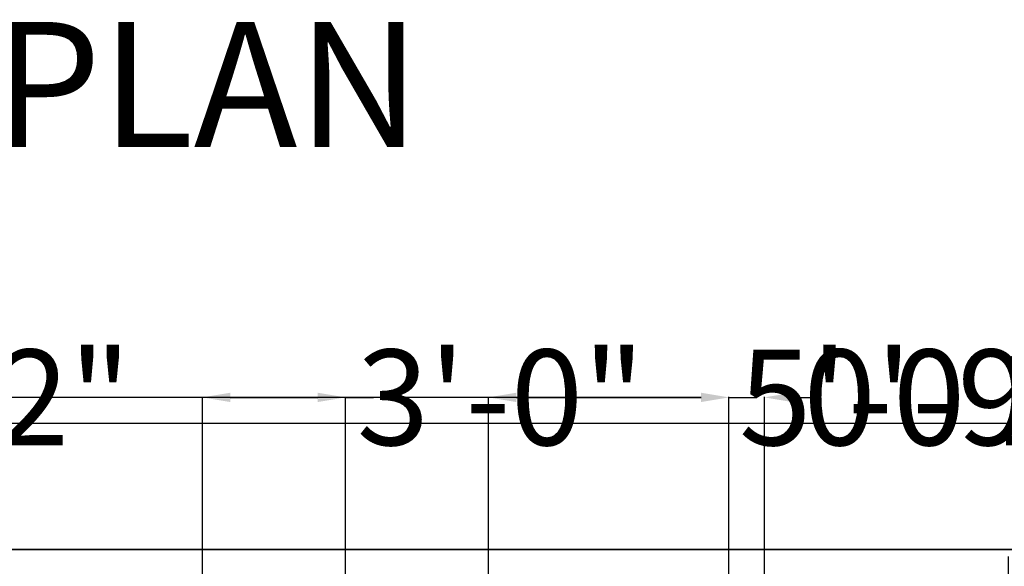
# Model space of a CAD drawing. Units: inches. Extents: x -166 to 1001, y 0 to 688.
# Tile 10 of 11: x 361 to 608, y 551 to 688. Entities that reach past the tile are written whole.
import ezdxf

# ---------------------------------------------------------------- set-up
doc = ezdxf.new("R2010")
doc.units = ezdxf.units.IN
doc.header["$MEASUREMENT"] = 0
for name, color, linetype, lineweight in [('A-ANNO-DIMS', 1, 'Continuous', 18), ('A-ANNO-TEXT', 2, 'Continuous', 25), ('C-SITE-WALL', 250, 'Continuous', 35)]:
    doc.layers.add(name, color=color, linetype=linetype, lineweight=lineweight)
doc.styles.get("Standard").update_dxf_attribs({"font": 'arial.ttf'})
doc.dimstyles.get("Standard").update_dxf_attribs({"dimtxt": 24, "dimasz": 7, "dimexe": 0.18, "dimexo": 0.0625, "dimgap": 0.09, "dimtad": 0, "dimtih": 1, "dimtoh": 1, "dimdec": 0, "dimzin": 0, "dimdsep": 46, "dimlunit": 3, "dimtxsty": 'Standard', "dimcen": 0.09, "dimadec": 0, "dimazin": 0, "dimtfac": 1, "dimtdec": 0, "dimtofl": 0, "dimtmove": 0, "dimatfit": 3, "dimfxl": 1, "dimtolj": 1, "dimtzin": 0, "dimarcsym": 0})

# ---------------------------------------------------------------- blocks, each defined once
blk = doc.blocks.new('*D10')
at = {"layer": 'A-ANNO-DIMS', "color": 0, "lineweight": -2, "transparency": 16777216}
for p, q in [((-82.62, 554.8), (-82.62, 586.48)), ((-75.62, 586.3), (256.61, 586.3)), ((629.88, 586.3), (297.65, 586.3)), ((636.88, 554.8), (636.88, 586.48))]:
    blk.add_line(p, q, dxfattribs=at)
at = {"layer": 'A-ANNO-DIMS', "color": 0, "transparency": 16777216}
for points in [[(-75.62, 587.47), (-75.62, 585.14), (-82.62, 586.3)], [(629.88, 587.47), (629.88, 585.14), (636.88, 586.3)]]:
    blk.add_solid(points, dxfattribs=at)
at = {"layer": 'Defpoints', "color": 0, "transparency": 16777216}
for p in [(636.88, 586.3), (-82.62, 554.74), (636.88, 554.74)]:
    blk.add_point(p, dxfattribs=at)
at = {"layer": 'A-ANNO-DIMS', "color": 0, "transparency": 16777216, "insert": (277.13, 586.3), "char_height": 24, "attachment_point": 5}
blk.add_mtext("\\A1;60'", dxfattribs=at)
blk = doc.blocks.new('*D15')
at = {"layer": 'A-ANNO-DIMS', "color": 0, "lineweight": -2, "transparency": 16777216}
for p, q in [((566.06, 508.76), (566.06, 503.04)), ((603.45, 508.76), (603.45, 503.04)), ((573.06, 503.22), (596.45, 503.22)), ((603.45, 503.22), (610.45, 503.22))]:
    blk.add_line(p, q, dxfattribs=at)
at = {"layer": 'A-ANNO-DIMS', "color": 0, "transparency": 16777216}
for points in [[(573.06, 504.38), (573.06, 502.05), (566.06, 503.22)], [(596.45, 504.38), (596.45, 502.05), (603.45, 503.22)]]:
    blk.add_solid(points, dxfattribs=at)
at = {"layer": 'Defpoints', "color": 0, "transparency": 16777216}
for p in [(566.06, 508.83), (603.45, 508.83), (603.45, 503.22)]:
    blk.add_point(p, dxfattribs=at)
at = {"layer": 'A-ANNO-DIMS', "color": 0, "transparency": 16777216, "insert": (774.93, 503.22), "char_height": 24, "attachment_point": 5}
blk.add_mtext('\\A1;SHRUB 3\'-1 1/2" TYP.', dxfattribs=at)
blk = doc.blocks.new('*D16')
at = {"layer": 'A-ANNO-DIMS', "color": 0, "lineweight": -2, "transparency": 16777216}
for p, q in [((609.06, 546), (609.06, 553)), ((603.51, 539), (609.24, 539)), ((603.51, 508.83), (609.24, 508.83)), ((609.06, 501.83), (609.06, 494.83))]:
    blk.add_line(p, q, dxfattribs=at)
at = {"layer": 'A-ANNO-DIMS', "color": 0, "transparency": 16777216}
for points in [[(607.89, 546), (610.23, 546), (609.06, 539)], [(607.89, 501.83), (610.23, 501.83), (609.06, 508.83)]]:
    blk.add_solid(points, dxfattribs=at)
at = {"layer": 'Defpoints', "color": 0, "transparency": 16777216}
for p in [(603.45, 539), (609.06, 539), (603.45, 508.83)]:
    blk.add_point(p, dxfattribs=at)
at = {"layer": 'A-ANNO-DIMS', "color": 0, "transparency": 16777216, "insert": (609.06, 523.91), "char_height": 24, "attachment_point": 5}
blk.add_mtext('\\A1;2\'-6" TYP.', dxfattribs=at)
blk = doc.blocks.new('*D35')
at = {"layer": 'A-ANNO-DIMS', "color": 0, "lineweight": -2, "transparency": 16777216}
for p, q in [((15.38, 483.8), (15.38, 593.07)), ((22.38, 592.89), (207.38, 592.89)), ((531.88, 592.89), (346.89, 592.89)), ((538.88, 483.8), (538.88, 593.07))]:
    blk.add_line(p, q, dxfattribs=at)
at = {"layer": 'A-ANNO-DIMS', "color": 0, "transparency": 16777216}
for points in [[(22.38, 594.06), (22.38, 591.72), (15.38, 592.89)], [(531.88, 594.06), (531.88, 591.72), (538.88, 592.89)]]:
    blk.add_solid(points, dxfattribs=at)
at = {"layer": 'Defpoints', "color": 0, "transparency": 16777216}
for p in [(538.88, 592.89), (15.38, 483.74), (538.88, 483.74)]:
    blk.add_point(p, dxfattribs=at)
at = {"layer": 'A-ANNO-DIMS', "color": 0, "transparency": 16777216, "insert": (277.13, 592.89), "char_height": 24, "attachment_point": 5}
blk.add_mtext('\\A1;43\'-7 1/2"', dxfattribs=at)
blk = doc.blocks.new('*D47')
at = {"layer": 'A-ANNO-DIMS', "color": 0, "lineweight": -2, "transparency": 16777216}
for p, q in [((478.46, 483.8), (478.46, 593.07)), ((485.46, 592.89), (531.88, 592.89)), ((538.88, 483.8), (538.88, 593.07)), ((538.88, 592.89), (545.88, 592.89))]:
    blk.add_line(p, q, dxfattribs=at)
at = {"layer": 'A-ANNO-DIMS', "color": 0, "transparency": 16777216}
for points in [[(485.46, 594.06), (485.46, 591.72), (478.46, 592.89)], [(531.88, 594.06), (531.88, 591.72), (538.88, 592.89)]]:
    blk.add_solid(points, dxfattribs=at)
at = {"layer": 'Defpoints', "color": 0, "transparency": 16777216}
for p in [(538.88, 592.89), (478.46, 483.74), (538.88, 483.74)]:
    blk.add_point(p, dxfattribs=at)
at = {"layer": 'A-ANNO-DIMS', "color": 0, "transparency": 16777216, "insert": (605.83, 592.89), "char_height": 24, "attachment_point": 5}
blk.add_mtext('\\A1;5\'-0 1/2"', dxfattribs=at)
blk = doc.blocks.new('*D57')
at = {"layer": 'A-ANNO-DIMS', "color": 0, "lineweight": -2, "transparency": 16777216}
for p, q in [((531.88, 592.89), (524.88, 592.89)), ((538.88, 335.97), (538.88, 593.07)), ((547.76, 325.77), (547.76, 593.07)), ((554.76, 592.89), (561.76, 592.89))]:
    blk.add_line(p, q, dxfattribs=at)
at = {"layer": 'A-ANNO-DIMS', "color": 0, "transparency": 16777216}
for points in [[(531.88, 594.06), (531.88, 591.72), (538.88, 592.89)], [(554.76, 594.06), (554.76, 591.72), (547.76, 592.89)]]:
    blk.add_solid(points, dxfattribs=at)
at = {"layer": 'Defpoints', "color": 0, "transparency": 16777216}
for p in [(547.76, 592.89), (538.88, 335.91), (547.76, 325.71)]:
    blk.add_point(p, dxfattribs=at)
at = {"layer": 'A-ANNO-DIMS', "color": 0, "transparency": 16777216, "insert": (593.75, 592.89), "char_height": 24, "attachment_point": 5}
blk.add_mtext('\\A1;0\'-9"', dxfattribs=at)
blk = doc.blocks.new('*D62')
at = {"layer": 'A-ANNO-DIMS', "color": 0, "lineweight": -2, "transparency": 16777216}
for p, q in [((201.55, 342.8), (201.55, 593.07)), ((208.55, 592.89), (249.88, 592.89)), ((256.88, 342.8), (256.88, 593.07)), ((256.88, 592.89), (263.88, 592.89))]:
    blk.add_line(p, q, dxfattribs=at)
at = {"layer": 'A-ANNO-DIMS', "color": 0, "transparency": 16777216}
for points in [[(208.55, 594.06), (208.55, 591.72), (201.55, 592.89)], [(249.88, 594.06), (249.88, 591.72), (256.88, 592.89)]]:
    blk.add_solid(points, dxfattribs=at)
at = {"layer": 'Defpoints', "color": 0, "transparency": 16777216}
for p in [(256.88, 592.89), (201.55, 342.74), (256.88, 342.74)]:
    blk.add_point(p, dxfattribs=at)
at = {"layer": 'A-ANNO-DIMS', "color": 0, "transparency": 16777216, "insert": (324.32, 592.89), "char_height": 24, "attachment_point": 5}
blk.add_mtext('\\A1;4\'-7 1/2"', dxfattribs=at)
blk = doc.blocks.new('*D71')
at = {"layer": 'A-ANNO-DIMS', "color": 0, "lineweight": -2, "transparency": 16777216}
for p, q in [((406.66, 278.3), (406.66, 593.07)), ((413.66, 592.89), (435.61, 592.89)), ((442.61, 278.3), (442.61, 593.07)), ((442.61, 592.89), (449.61, 592.89))]:
    blk.add_line(p, q, dxfattribs=at)
at = {"layer": 'A-ANNO-DIMS', "color": 0, "transparency": 16777216}
for points in [[(413.66, 594.06), (413.66, 591.72), (406.66, 592.89)], [(435.61, 594.06), (435.61, 591.72), (442.61, 592.89)]]:
    blk.add_solid(points, dxfattribs=at)
at = {"layer": 'Defpoints', "color": 0, "transparency": 16777216}
for p in [(442.61, 592.89), (406.66, 278.24), (442.61, 278.24)]:
    blk.add_point(p, dxfattribs=at)
at = {"layer": 'A-ANNO-DIMS', "color": 0, "transparency": 16777216, "insert": (481.59, 592.89), "char_height": 24, "attachment_point": 5}
blk.add_mtext('\\A1;3\'-0"', dxfattribs=at)

msp = doc.modelspace()

# ---------------------------------------------------------------- linework, layer by layer
at = {"layer": 'C-SITE-WALL'}
msp.add_line((-82.62, 554.74), (636.88, 554.74), dxfattribs=at)

# ---------------------------------------------------------------- texts
at = {"layer": 'A-ANNO-TEXT'}
msp.add_text('GROUND FLOOR PLAN', height=31.3778, dxfattribs=at).set_placement((17.68, 655.72))

# ---------------------------------------------------------------- dimensions: what is measured, and where the dimension line sits
at = {"layer": 'A-ANNO-DIMS'}
for base, p1, p2, override, picture, middle in [((538.88, 592.89), (15.38, 483.74), (538.88, 483.74), {"dimdec": 1, "dimlfac": 1, "dimrnd": 0, "dimzin": 1, "dimdsep": 46, "dimlunit": 4, "dimfrac": 2}, '*D35', (277.13, 592.89)), ((256.88, 592.89), (201.55, 342.74), (256.88, 342.74), {"dimdec": 1, "dimlfac": 1, "dimrnd": 0, "dimzin": 1, "dimdsep": 46, "dimlunit": 4, "dimfrac": 2}, '*D62', (324.32, 592.89)), ((538.88, 592.89), (478.46, 483.74), (538.88, 483.74), {"dimdec": 1, "dimlfac": 1, "dimrnd": 0, "dimzin": 1, "dimdsep": 46, "dimlunit": 4, "dimfrac": 2}, '*D47', (605.83, 592.89)), ((442.6082, 592.8909), (406.6614, 278.2409), (442.6082, 278.2409), {"dimdec": 1, "dimlfac": 1, "dimrnd": 0, "dimzin": 1, "dimdsep": 46, "dimlunit": 4, "dimfrac": 2}, '*D71', (481.589, 592.8909)), ((547.76, 592.89), (538.88, 335.91), (547.76, 325.71), {"dimdec": 1, "dimlfac": 1, "dimrnd": 0, "dimzin": 1, "dimdsep": 46, "dimlunit": 4, "dimfrac": 2}, '*D57', (593.75, 592.89)), ((636.88246038, 586.30455527), (-82.61753962, 554.740867), (636.88246038, 554.740867), {"dimclrd": 0, "dimclre": 0, "dimclrt": 0}, '*D10', (277.13246038, 586.30455527))]:
    dim = msp.add_linear_dim(base=base, p1=p1, p2=p2, dimstyle='Standard', override=override, dxfattribs=at)
    dim.commit()
    dim.dimension.update_dxf_attribs({"geometry": picture, "text_midpoint": middle})
dim = msp.add_linear_dim(base=(603.45, 503.22), p1=(566.06, 508.83), p2=(603.45, 508.83), text='SHRUB <> TYP.', dimstyle='Standard', override={"dimdec": 1, "dimlfac": 1, "dimrnd": 0, "dimzin": 1, "dimdsep": 46, "dimlunit": 4, "dimfrac": 2}, dxfattribs=at)
dim.commit()
dim.dimension.update_dxf_attribs({"geometry": '*D15', "text_midpoint": (774.93, 503.22)})
dim = msp.add_linear_dim(base=(609.06, 539), p1=(603.45, 508.83), p2=(603.45, 539), angle=90, text='<> TYP.', dimstyle='Standard', override={"dimdec": 1, "dimlfac": 1, "dimrnd": 0, "dimzin": 1, "dimdsep": 46, "dimlunit": 4, "dimfrac": 2}, dxfattribs=at)
dim.commit()
dim.dimension.update_dxf_attribs({"geometry": '*D16', "text_midpoint": (609.06, 523.91)})

doc.saveas('drawing.dxf')
